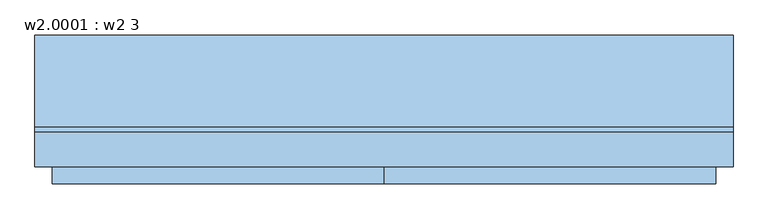
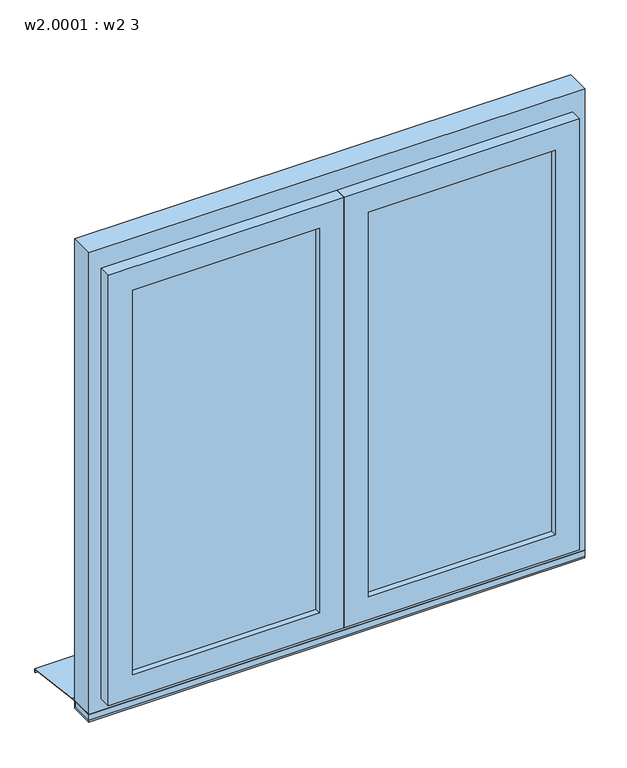
"""IFC4 building model written with IfcOpenShell, lengths in millimetres: window geometry, w2.0001 : w2 3."""

from ifc_helpers import new_model, si_unit, frame, origin, place, context, project, spatial, polyline, outline, extrude, faceted_brep, source, transform, mapped, element, save


def w2_0001_w2_3_7b164e2c(model_context):
    return source(origin(), model_context, "Body", "SolidModel", [
        extrude(outline(polyline([(-72.8278457, 1020.0), (87.15, 1000.0), (87.15, 990.0), (85.15, 990.0), (85.15, 998.3604634), (-73.0259277, 1018.0), (-82.85, 1018.0), (-82.85, 1020.0), (-72.8278457, 1020.0)])), frame((-609.6, 0.0, 0.0), z_axis=(1.0, 0.0, 0.0), x_axis=(0.0, 1.0, 0.0)), (0.0, 0.0, 1.0), 1219.2),
        extrude(outline(polyline([(-609.6, -142.85), (-609.6, -87.15), (609.6, -87.15), (609.6, -142.85), (-609.6, -142.85)])), frame((0.0, 0.0, 1005.0), z_axis=(0.0, 0.0, 1.0), x_axis=(1.0, 0.0, 0.0)), (0.0, 0.0, 1.0), 15.0),
        extrude(outline(polyline([(60.0, -127.85), (519.6, -127.85), (519.6, -157.85), (60.0, -157.85), (60.0, -127.85)])), frame((0.0, 0.0, 1110.0), z_axis=(0.0, 0.0, 1.0), x_axis=(1.0, 0.0, 0.0)), (0.0, 0.0, 1.0), 999.2),
        extrude(outline(polyline([(-519.6, -127.85), (-60.0, -127.85), (-60.0, -157.85), (-519.6, -157.85), (-519.6, -127.85)])), frame((0.0, 0.0, 1110.0), z_axis=(0.0, 0.0, 1.0), x_axis=(1.0, 0.0, 0.0)), (0.0, 0.0, 1.0), 999.2),
        extrude(outline(polyline([(2219.2, -609.6), (1000.0, -609.6), (1000.0, 609.6), (2219.2, 609.6), (2219.2, -609.6)]), holes=[polyline([(2139.2, -549.6), (2139.2, 549.6), (1080.0, 549.6), (1080.0, -549.6), (2139.2, -549.6)])]), frame((0.0, -142.85, 0.0), z_axis=(0.0, 1.0, 0.0), x_axis=(0.0, 0.0, 1.0)), (0.0, 0.0, 1.0), 60.0),
        extrude(outline(polyline([(30.0, -142.85), (-30.0, -142.85), (-30.0, -82.85), (30.0, -82.85), (30.0, -142.85)])), frame((0.0, 0.0, 1080.0), z_axis=(0.0, 0.0, 1.0), x_axis=(1.0, 0.0, 0.0)), (0.0, 0.0, 1.0), 1059.2),
        faceted_brep([(30.0, -142.85, 1080.0), (30.0, -112.85, 1080.0), (549.6, -112.85, 1080.0), (549.6, -142.85, 1080.0), (549.6, -112.85, 2139.2), (549.6, -142.85, 2139.2), (30.0, -112.85, 2139.2), (519.6, -112.85, 2109.2), (60.0, -112.85, 2109.2), (60.0, -112.85, 1110.0), (519.6, -112.85, 1110.0), (579.6, -142.85, 1050.0), (0.0, -142.85, 1050.0), (0.0, -142.85, 2169.2), (579.6, -142.85, 2169.2), (30.0, -142.85, 2139.2), (0.0, -172.85, 1050.0), (579.6, -172.85, 1050.0), (579.6, -172.85, 2169.2), (0.0, -172.85, 2169.2), (519.6, -172.85, 1110.0), (60.0, -172.85, 1110.0), (60.0, -172.85, 2109.2), (519.6, -172.85, 2109.2)], [[[0, 1, 2, 3]], [[3, 2, 4, 5]], [[2, 1, 6, 4], [7, 8, 9, 10]], [[11, 12, 13, 14], [5, 15, 0, 3]], [[16, 12, 11, 17]], [[17, 11, 14, 18]], [[18, 19, 16, 17], [20, 21, 22, 23]], [[9, 21, 20, 10]], [[10, 20, 23, 7]], [[15, 6, 1, 0]], [[19, 13, 12, 16]], [[8, 22, 21, 9]], [[5, 4, 6, 15]], [[18, 14, 13, 19]], [[7, 23, 22, 8]]]),
        faceted_brep([(-549.6, -142.85, 1080.0), (-549.6, -112.85, 1080.0), (-30.0, -112.85, 1080.0), (-30.0, -142.85, 1080.0), (-30.0, -112.85, 2139.2), (-30.0, -142.85, 2139.2), (-549.6, -112.85, 2139.2), (-60.0, -112.85, 2109.2), (-519.6, -112.85, 2109.2), (-519.6, -112.85, 1110.0), (-60.0, -112.85, 1110.0), (0.0, -142.85, 1050.0), (-579.6, -142.85, 1050.0), (-579.6, -142.85, 2169.2), (0.0, -142.85, 2169.2), (-549.6, -142.85, 2139.2), (-579.6, -172.85, 1050.0), (0.0, -172.85, 1050.0), (0.0, -172.85, 2169.2), (-579.6, -172.85, 2169.2), (-60.0, -172.85, 1110.0), (-519.6, -172.85, 1110.0), (-519.6, -172.85, 2109.2), (-60.0, -172.85, 2109.2)], [[[0, 1, 2, 3]], [[3, 2, 4, 5]], [[2, 1, 6, 4], [7, 8, 9, 10]], [[11, 12, 13, 14], [5, 15, 0, 3]], [[16, 12, 11, 17]], [[17, 11, 14, 18]], [[18, 19, 16, 17], [20, 21, 22, 23]], [[9, 21, 20, 10]], [[10, 20, 23, 7]], [[15, 6, 1, 0]], [[19, 13, 12, 16]], [[8, 22, 21, 9]], [[5, 4, 6, 15]], [[18, 14, 13, 19]], [[7, 23, 22, 8]]]),
    ])


if __name__ == "__main__":
    model = new_model("IFC4")
    model_context = context("Model", 3, world=origin())
    ifc_project = project(units=[si_unit("LENGTHUNIT", "METRE", prefix="MILLI")], contexts=[model_context])
    site = spatial("IfcSite", under=ifc_project)
    building = spatial("IfcBuilding", under=site)
    placement = place(None, origin())
    w2_0001_w2_3_shape = w2_0001_w2_3_7b164e2c(model_context)
    element("IfcWindow", 1, ObjectType="w2.0001 : w2 3", at=placement, inside=building, context=model_context, shape_type="MappedRepresentation", body=[
        mapped(w2_0001_w2_3_shape, transform((0.0, 0.0, 0.0), x_axis=(1.0, 0.0, 0.0), y_axis=(0.0, 1.0, 0.0), z_axis=(0.0, 0.0, 1.0))),
    ])
    save(model, "model.ifc")

# Revit data of these elements
# Type "w2.0001 : w2 3"
#   Type Mark = "21"
#   Operation = "DoublePanelVertical"
#   Keynote = "16.05.01"
#   Analytic Construction = "<None>"
#   Rough Width = 4' - 0"
#   Rough Height = 4' - 0"
#   Rahmentiefe = 0' - 2.3622"
#   Rahmenhöhe unten = 0' - 3.14961"
#   Rahmehöhe oben = 0' - 3.14961"
#   Rahmenbreite = 0' - 2.3622"
#   Height = 4' - 0"
#   Flügeltiefe = 0' - 2.3622"
#   Flügelbreite = 0' - 2.3622"
#   Einbautiefe (von außen) [instance default] = 0' - 5.51181"
#   Width = 4' - 0"
#   Kippflügel [instance default] = yes
#   Drehflügel im Grundriß darstellen [instance default] = no
#   Drehflügel [instance default] = yes
#   Define Thermal Properties by = 1
#   Rahmen [instance default] = none
#   Glas [instance default] = none
#   Flügel [instance default] = none
#   Fensterbank aussen [instance default] = none
#   Fensterbank innen [instance default] = none
#   Wall Closure = (empty or 0)
# Element 1 (IfcWindow, "w2.0001 : w2 3")
#   Materials on its faces: "Fenster - Kunststoff", "Fenster - Kunststoff weiss", "Glass", "Fenster - Holz"
# Materials
#   "Fenster - Kunststoff": colour RGB 249 249 249, transparency 0
#   "Fenster - Kunststoff weiss": colour RGB 249 249 249, transparency 0
#   "Glass": class "Glass", colour RGB 0 128 192, transparency 0.75, Description = "Soda Lime Glass", Cost = 0
#   "Fenster - Holz": colour RGB 216 135 75, transparency 0
